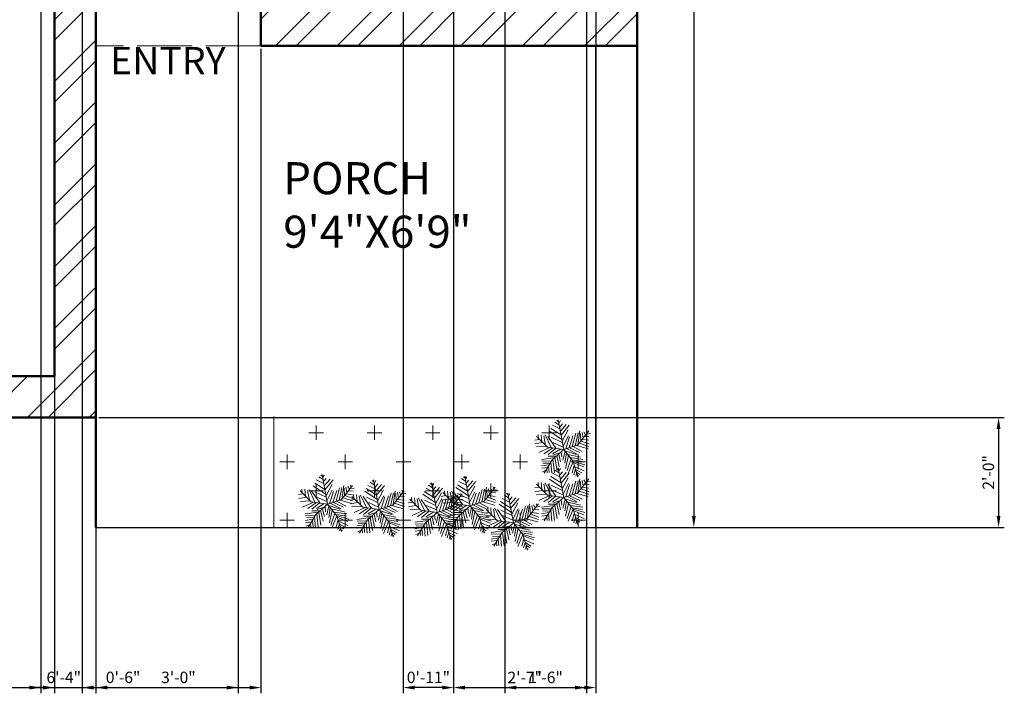
# Model space of a CAD drawing. Units: inches. Extents: x 1147 to 1568, y 1982 to 2559.
# Tile 2 of 4: x 1353 to 1568, y 1982 to 2128. Entities that reach past the tile are written whole.
import ezdxf

# ---------------------------------------------------------------- set-up
doc = ezdxf.new("R2010")
doc.units = ezdxf.units.IN
doc.linetypes.add('ACAD_ISO02W100', pattern=[15, 12, -3])
for name, color, linetype, lineweight in [('A-ANNO-DIMS', 2, 'Continuous', 18), ('A-FLOR', 7, 'Continuous', 25), ('A-WALL', 7, 'Continuous', 50), ('A-WALL-PATT', 252, 'Continuous', 13), ('L-PLNT', 3, 'Continuous', 18)]:
    doc.layers.add(name, color=color, linetype=linetype, lineweight=lineweight)
for name, color, linetype, lineweight, true_color in [('A-ANNO-TEXT', 244, 'Continuous', 18, 0x991b1e), ('A-AREA-IDEN', 244, 'Continuous', 25, 0x991b1e), ('A-WALL-OVHD', 244, 'ACAD_ISO02W100', 18, 0x991b1e), ('L-PLNT-PATT', 116, 'Continuous', 13, 0x136734)]:
    doc.layers.add(name, color=color, linetype=linetype, lineweight=lineweight, true_color=true_color)
doc.styles.get("Standard").update_dxf_attribs({"font": 'arial.ttf'})
doc.dimstyles.new('ISO-25', dxfattribs={"dimtxt": 2.5, "dimasz": 2.5, "dimexe": 1.25, "dimexo": 0.625, "dimtad": 1, "dimlunit": 3, "dimtxsty": 'Standard', "dimcen": 2.5, "dimadec": 0, "dimazin": 0, "dimtfac": 1, "dimtmove": 0, "dimatfit": 3, "dimfxl": 1, "dimarcsym": 0})

# ---------------------------------------------------------------- blocks, each defined once
blk = doc.blocks.new('*U8')
for p, q in [((0, 0), (-10.5, 57)), ((-5.114, 28.097), (-24.676, 40.636)), ((-7.288, 39.707), (-21.778, 46.673)), ((-8.737, 47.138), (-17.069, 52.711)), ((-10.186, 53.64), (-13.084, 55.962)), ((-9.099, 51.782), (-6.563, 55.962)), ((-7.65, 43.423), (-2.578, 49.46)), ((-5.839, 35.992), (4.667, 48.067)), ((-5.114, 27.632), (10.463, 46.673)), ((-2.941, 16.486), (8.652, 37.85)), ((-47.498, 19.737), (-55.83, 18.344)), ((-31.5, 4.5), (-52.5, 25.5)), ((-48.585, 21.131), (-49.309, 29.026)), ((-43.513, 28.561), (-42.427, 15.558)), ((-38.442, 26.239), (-34.819, 7.663)), ((-35.544, 28.097), (-24.314, 3.947)), ((-14.533, 2.09), (-30.834, 25.31)), ((-3.665, 19.273), (-27.574, 35.527)), ((-24.314, 23.917), (-2.941, 13.7)), ((-1.129, 6.734), (9.014, 26.704)), ((3.942, 1.625), (11.187, 24.381)), ((10.101, 3.483), (17.708, 26.239)), ((16.259, 5.805), (23.142, 31.348)), ((22.055, 7.198), (27.489, 32.277)), ((27, 9), (48, 36)), ((27.127, 9.056), (31.112, 35.992)), ((31.836, 30.883), (32.561, 16.486)), ((35.096, 32.741), (37.27, 22.524)), ((36.183, 19.737), (48.137, 17.88)), ((38.719, 34.134), (41.979, 28.561)), ((40.53, 25.775), (48.862, 24.846)), ((43.791, 29.954), (51.036, 30.883)), ((44.153, 36.456), (45.239, 32.741)), ((-40.615, 13.7), (-55.105, 10.913)), ((-33.37, 6.269), (-52.207, 5.34)), ((-28.299, 3.483), (-47.86, -5.805)), ((-21.416, 3.018), (-38.079, -8.128)), ((0, 0), (-31.5, 4.5)), ((-15.982, 2.09), (-30.11, -9.521)), ((0, 0), (-22.5, -19.5)), ((-6.563, 1.161), (-21.416, -8.128)), ((-20.691, 13.7), (-1.129, 4.876)), ((0, 0), (27, 9)), ((0, 0), (18, -22.5)), ((6.478, 1.625), (26.04, -8.592)), ((11.187, 3.483), (30.749, -5.805)), ((18.07, 5.805), (35.096, -3.483)), ((24.229, 7.663), (46.688, 1.625)), ((29.662, 12.307), (48.137, 6.269)), ((33.285, 16.486), (48.862, 10.913)), ((-17.431, -15.094), (-42.789, -18.809)), ((-15.257, -12.772), (-30.11, -12.772)), ((-20.691, -18.345), (-17.793, -44.352)), ((-6.563, -5.805), (-19.967, -9.985)), ((-17.069, -15.094), (-12.721, -40.172)), ((-13.446, -11.378), (-8.737, -32.741)), ((-9.461, -8.592), (-6.201, -23.453)), ((-4.752, -3.483), (-3.665, -14.629)), ((2.493, -3.019), (-1.491, -20.202)), ((1.769, -2.555), (24.229, -9.521)), ((5.029, -6.27), (2.131, -25.775)), ((9.014, -11.378), (3.58, -35.992)), ((14.085, -16.951), (6.478, -40.172)), ((7.565, -9.056), (32.198, -14.629)), ((12.274, -15.094), (36.907, -18.809)), ((-28.299, -29.026), (-42.789, -31.348)), ((-24.314, -21.596), (-42.427, -22.06)), ((-30.834, -34.135), (-42.427, -35.528)), ((-26.849, -26.24), (-40.253, -25.775)), ((-22.5, -19.5), (-37.5, -45)), ((-32.646, -36.921), (-31.921, -44.352)), ((-29.023, -30.884), (-27.936, -43.887)), ((-25.038, -23.918), (-22.865, -45.281)), ((18.07, -22.524), (8.289, -45.745)), ((20.244, -30.419), (15.897, -44.816)), ((16.259, -19.738), (36.183, -22.989)), ((18, -22.5), (27, -52.5)), ((18.433, -22.524), (40.53, -29.026)), ((19.157, -25.311), (38.719, -33.206)), ((21.331, -32.741), (39.081, -40.636)), ((-34.457, -39.708), (-40.978, -42.494)), ((22.78, -37.85), (19.519, -48.532)), ((22.78, -38.314), (34.372, -44.816)), ((24.591, -45.745), (23.142, -50.854)), ((24.591, -43.423), (30.749, -47.603)), ((26.764, -49.925), (28.213, -50.854))]:
    blk.add_line(p, q)
blk = doc.blocks.new('*D13')
at = {"layer": 'A-ANNO-DIMS', "color": 0, "lineweight": -2, "transparency": 16777216}
for p, q in [((1488.23, 2527.7), (1501.22, 2527.7)), ((1499.97, 2525.2), (1499.97, 2020.2)), ((1488.23, 2017.7), (1501.22, 2017.7))]:
    blk.add_line(p, q, dxfattribs=at)
at = {"layer": 'A-ANNO-DIMS', "color": 0, "transparency": 16777216}
for points in [[(1499.56, 2525.2), (1500.39, 2525.2), (1499.97, 2527.7)], [(1499.56, 2020.2), (1500.39, 2020.2), (1499.97, 2017.7)]]:
    blk.add_solid(points, dxfattribs=at)
at = {"layer": 'Defpoints', "color": 0, "transparency": 16777216}
for p in [(1487.61, 2527.7), (1487.61, 2017.7), (1499.97, 2017.7)]:
    blk.add_point(p, dxfattribs=at)
at = {"layer": 'A-ANNO-DIMS', "color": 0, "transparency": 16777216, "insert": (1498.07, 2272.7), "char_height": 2.5, "attachment_point": 5, "rotation": 90}
blk.add_mtext('42\'-6"', dxfattribs=at)
blk = doc.blocks.new('*D43')
at = {"layer": 'A-ANNO-DIMS', "color": 0, "lineweight": -2, "transparency": 16777216}
for p, q in [((1327.61, 2368.08), (1327.61, 1981.52)), ((1357.61, 2368.08), (1357.61, 1981.52)), ((1330.11, 1982.77), (1355.11, 1982.77))]:
    blk.add_line(p, q, dxfattribs=at)
at = {"layer": 'A-ANNO-DIMS', "color": 0, "transparency": 16777216}
for points in [[(1330.11, 1983.19), (1330.11, 1982.35), (1327.61, 1982.77)], [(1355.11, 1983.19), (1355.11, 1982.35), (1357.61, 1982.77)]]:
    blk.add_solid(points, dxfattribs=at)
at = {"layer": 'Defpoints', "color": 0, "transparency": 16777216}
for p in [(1327.61, 2368.7), (1357.61, 2368.7), (1357.61, 1982.77)]:
    blk.add_point(p, dxfattribs=at)
at = {"layer": 'A-ANNO-DIMS', "color": 0, "transparency": 16777216, "insert": (1342.61, 1984.67), "char_height": 2.5, "attachment_point": 5}
blk.add_mtext('2\'-6"', dxfattribs=at)
blk = doc.blocks.new('*D46')
at = {"layer": 'A-ANNO-DIMS', "color": 0, "lineweight": -2, "transparency": 16777216}
for p, q in [((1369.61, 2122.08), (1369.61, 1981.52)), ((1405.61, 2122.08), (1405.61, 1981.52)), ((1372.11, 1982.77), (1403.11, 1982.77))]:
    blk.add_line(p, q, dxfattribs=at)
at = {"layer": 'A-ANNO-DIMS', "color": 0, "transparency": 16777216}
for points in [[(1372.11, 1983.19), (1372.11, 1982.35), (1369.61, 1982.77)], [(1403.11, 1983.19), (1403.11, 1982.35), (1405.61, 1982.77)]]:
    blk.add_solid(points, dxfattribs=at)
at = {"layer": 'Defpoints', "color": 0, "transparency": 16777216}
for p in [(1369.61, 2122.7), (1405.61, 2122.7), (1405.61, 1982.77)]:
    blk.add_point(p, dxfattribs=at)
at = {"layer": 'A-ANNO-DIMS', "color": 0, "transparency": 16777216, "insert": (1387.61, 1984.67), "char_height": 2.5, "attachment_point": 5}
blk.add_mtext('3\'-0"', dxfattribs=at)
blk = doc.blocks.new('*D47')
at = {"layer": 'A-ANNO-DIMS', "color": 0, "lineweight": -2, "transparency": 16777216}
for p, q in [((1436.61, 2166.08), (1436.61, 1981.52)), ((1447.61, 2166.08), (1447.61, 1981.52)), ((1445.11, 1982.77), (1439.11, 1982.77))]:
    blk.add_line(p, q, dxfattribs=at)
at = {"layer": 'A-ANNO-DIMS', "color": 0, "transparency": 16777216}
for points in [[(1439.11, 1983.19), (1439.11, 1982.35), (1436.61, 1982.77)], [(1445.11, 1983.19), (1445.11, 1982.35), (1447.61, 1982.77)]]:
    blk.add_solid(points, dxfattribs=at)
at = {"layer": 'Defpoints', "color": 0, "transparency": 16777216}
for p in [(1436.61, 2166.7), (1447.61, 2166.7), (1436.61, 1982.77)]:
    blk.add_point(p, dxfattribs=at)
at = {"layer": 'A-ANNO-DIMS', "color": 0, "transparency": 16777216, "insert": (1442.11, 1984.67), "char_height": 2.5, "attachment_point": 5}
blk.add_mtext('0\'-11"', dxfattribs=at)
blk = doc.blocks.new('*D49')
at = {"layer": 'A-ANNO-DIMS', "color": 0, "lineweight": -2, "transparency": 16777216}
for p, q in [((1447.61, 2131.08), (1447.61, 1981.52)), ((1478.61, 2131.08), (1478.61, 1981.52)), ((1450.11, 1982.77), (1476.11, 1982.77))]:
    blk.add_line(p, q, dxfattribs=at)
at = {"layer": 'A-ANNO-DIMS', "color": 0, "transparency": 16777216}
for points in [[(1450.11, 1983.19), (1450.11, 1982.35), (1447.61, 1982.77)], [(1476.11, 1983.19), (1476.11, 1982.35), (1478.61, 1982.77)]]:
    blk.add_solid(points, dxfattribs=at)
at = {"layer": 'Defpoints', "color": 0, "transparency": 16777216}
for p in [(1447.61, 2131.7), (1478.61, 2131.7), (1478.61, 1982.77)]:
    blk.add_point(p, dxfattribs=at)
at = {"layer": 'A-ANNO-DIMS', "color": 0, "transparency": 16777216, "insert": (1463.11, 1984.65), "char_height": 2.5, "attachment_point": 5}
blk.add_mtext('2\'-7"', dxfattribs=at)
blk = doc.blocks.new('*D51')
at = {"layer": 'A-ANNO-DIMS', "color": 0, "lineweight": -2, "transparency": 16777216}
for p, q in [((1360.61, 2518.08), (1360.61, 1981.52)), ((1366.61, 2518.08), (1366.61, 1981.52)), ((1358.11, 1982.77), (1355.61, 1982.77)), ((1360.61, 1982.77), (1366.61, 1982.77)), ((1369.11, 1982.77), (1379.5, 1982.77))]:
    blk.add_line(p, q, dxfattribs=at)
at = {"layer": 'A-ANNO-DIMS', "color": 0, "transparency": 16777216}
for points in [[(1358.11, 1983.19), (1358.11, 1982.35), (1360.61, 1982.77)], [(1369.11, 1983.19), (1369.11, 1982.35), (1366.61, 1982.77)]]:
    blk.add_solid(points, dxfattribs=at)
at = {"layer": 'Defpoints', "color": 0, "transparency": 16777216}
for p in [(1360.61, 2518.7), (1366.61, 2518.7), (1366.61, 1982.77)]:
    blk.add_point(p, dxfattribs=at)
at = {"layer": 'A-ANNO-DIMS', "color": 0, "transparency": 16777216, "insert": (1375.55, 1984.67), "char_height": 2.5, "attachment_point": 5}
blk.add_mtext('0\'-6"', dxfattribs=at)
blk = doc.blocks.new('*D56')
at = {"layer": 'A-ANNO-DIMS', "color": 0, "lineweight": -2, "transparency": 16777216}
for p, q in [((1370.23, 2041.7), (1567.66, 2041.7)), ((1566.41, 2039.2), (1566.41, 2020.2)), ((1370.23, 2017.7), (1567.66, 2017.7))]:
    blk.add_line(p, q, dxfattribs=at)
at = {"layer": 'A-ANNO-DIMS', "color": 0, "transparency": 16777216}
for points in [[(1565.99, 2039.2), (1566.82, 2039.2), (1566.41, 2041.7)], [(1565.99, 2020.2), (1566.82, 2020.2), (1566.41, 2017.7)]]:
    blk.add_solid(points, dxfattribs=at)
at = {"layer": 'Defpoints', "color": 0, "transparency": 16777216}
for p in [(1369.61, 2041.7), (1369.61, 2017.7), (1566.41, 2017.7)]:
    blk.add_point(p, dxfattribs=at)
at = {"layer": 'A-ANNO-DIMS', "color": 0, "transparency": 16777216, "insert": (1564.51, 2029.7), "char_height": 2.5, "attachment_point": 5, "rotation": 90}
blk.add_mtext('2\'-0"', dxfattribs=at)
blk = doc.blocks.new('*D62')
at = {"layer": 'A-ANNO-DIMS', "color": 0, "lineweight": -2, "transparency": 16777216}
for p, q in [((1324.61, 2335.08), (1324.61, 1981.52)), ((1400.61, 2335.08), (1400.61, 1981.52)), ((1327.11, 1982.77), (1398.11, 1982.77))]:
    blk.add_line(p, q, dxfattribs=at)
at = {"layer": 'A-ANNO-DIMS', "color": 0, "transparency": 16777216}
for points in [[(1327.11, 1983.19), (1327.11, 1982.35), (1324.61, 1982.77)], [(1398.11, 1983.19), (1398.11, 1982.35), (1400.61, 1982.77)]]:
    blk.add_solid(points, dxfattribs=at)
at = {"layer": 'Defpoints', "color": 0, "transparency": 16777216}
for p in [(1324.61, 2335.7), (1400.61, 2335.7), (1400.61, 1982.77)]:
    blk.add_point(p, dxfattribs=at)
at = {"layer": 'A-ANNO-DIMS', "color": 0, "transparency": 16777216, "insert": (1362.61, 1984.67), "char_height": 2.5, "attachment_point": 5}
blk.add_mtext('6\'-4"', dxfattribs=at)
blk = doc.blocks.new('*D65')
at = {"layer": 'A-ANNO-DIMS', "color": 0, "lineweight": -2, "transparency": 16777216}
for p, q in [((1458.78, 2235.1), (1458.78, 1981.52)), ((1476.55, 2235.16), (1476.55, 1981.52)), ((1461.28, 1982.77), (1474.05, 1982.77))]:
    blk.add_line(p, q, dxfattribs=at)
at = {"layer": 'A-ANNO-DIMS', "color": 0, "transparency": 16777216}
for points in [[(1461.28, 1983.19), (1461.28, 1982.35), (1458.78, 1982.77)], [(1474.05, 1983.19), (1474.05, 1982.35), (1476.55, 1982.77)]]:
    blk.add_solid(points, dxfattribs=at)
at = {"layer": 'Defpoints', "color": 0, "transparency": 16777216}
for p in [(1458.78, 2235.73), (1476.55, 2235.78), (1476.55, 1982.77)]:
    blk.add_point(p, dxfattribs=at)
at = {"layer": 'A-ANNO-DIMS', "color": 0, "transparency": 16777216, "insert": (1467.66, 1984.67), "char_height": 2.5, "attachment_point": 5}
blk.add_mtext('1\'-6"', dxfattribs=at)

msp = doc.modelspace()

# ---------------------------------------------------------------- hatches: boundary and pattern name
at = {"layer": 'A-WALL-PATT'}
h = msp.add_hatch(dxfattribs=at)
h.set_pattern_fill('ANSI32', color=256)
h.paths.add_polyline_path([(1240.607, 2518.704), (1268.63, 2518.704), (1268.63, 2527.704), (1231.607, 2527.704), (1231.607, 2348.295), (1240.607, 2348.295), (1240.607, 2368.704), (1318.607, 2368.704), (1318.607, 2365.704), (1324.607, 2365.704), (1324.607, 2368.704), (1327.607, 2368.704), (1327.607, 2374.704), (1240.607, 2374.704)])
h.paths.add_polyline_path([(1324.607, 2335.704), (1318.607, 2335.704), (1318.607, 2314.704), (1240.607, 2314.704), (1240.607, 2324.295), (1231.607, 2324.295), (1231.607, 2247.419), (1240.607, 2247.419), (1240.607, 2308.704), (1324.607, 2308.704)])
h.paths.add_polyline_path([(1487.607, 2527.704), (1464.679, 2527.704), (1464.679, 2518.704), (1478.607, 2518.704), (1478.607, 2374.704), (1399.607, 2374.704), (1399.607, 2368.704), (1400.607, 2368.704), (1400.607, 2365.704), (1406.607, 2365.704), (1406.607, 2368.704), (1478.607, 2368.704), (1478.607, 2343.549), (1487.607, 2343.549)])
h.paths.add_polyline_path([(1366.607, 2518.704), (1398.679, 2518.704), (1398.679, 2527.704), (1334.63, 2527.704), (1334.63, 2518.704), (1360.607, 2518.704), (1360.607, 2374.704), (1357.607, 2374.704), (1357.607, 2368.704), (1369.607, 2368.704), (1369.607, 2374.704), (1366.607, 2374.704)])
h.paths.add_polyline_path([(1487.607, 2319.549), (1478.607, 2319.549), (1478.607, 2314.704), (1406.607, 2314.704), (1406.607, 2335.704), (1400.607, 2335.704), (1400.607, 2308.704), (1406.607, 2308.704), (1406.607, 2284.704), (1412.607, 2284.704), (1412.607, 2308.704), (1478.607, 2308.704), (1478.607, 2295.917), (1487.607, 2295.917)])
h.paths.add_polyline_path([(1487.607, 2235.917), (1478.607, 2235.917), (1478.607, 2212.704), (1400.607, 2212.704), (1400.607, 2206.704), (1478.607, 2206.704), (1478.607, 2131.704), (1405.607, 2131.704), (1405.607, 2122.704), (1487.607, 2122.704)])
h.paths.add_polyline_path([(1369.607, 2122.704), (1369.607, 2131.704), (1366.607, 2131.704), (1366.607, 2176.704), (1357.607, 2176.704), (1357.607, 2170.704), (1360.607, 2170.704), (1360.607, 2050.704), (1334.63, 2050.704), (1334.63, 2041.704), (1369.607, 2041.704)])
h.paths.add_polyline_path([(1240.607, 2170.704), (1321.607, 2170.704), (1321.607, 2176.704), (1240.607, 2176.704), (1240.607, 2187.419), (1231.607, 2187.419), (1231.607, 2041.704), (1268.63, 2041.704), (1268.63, 2050.704), (1240.607, 2050.704)])
at = {"layer": 'L-PLNT-PATT'}
h = msp.add_hatch(dxfattribs=at)
h.set_pattern_fill('CROSS', color=256)
h.paths.add_polyline_path([(1478.607, 2041.704), (1408.398, 2041.704), (1408.398, 2017.704), (1478.607, 2017.704)])
h.paths.add_polyline_path([(1431.023, 2023.435), (1431.134, 2023.64), (1430.963, 2023.756)], flags=16)
h.paths.add_polyline_path([(1436.583, 2025.011), (1436.507, 2025.271), (1436.274, 2024.971)], flags=16)
h.paths.add_polyline_path([(1431.899, 2020.624), (1432.179, 2020.56), (1431.935, 2020.865)], flags=16)
h.paths.add_polyline_path([(1430.596, 2020.912), (1430.247, 2020.803), (1430.282, 2020.641)], flags=16)
h.paths.add_polyline_path([(1420.698, 2022.051), (1420.662, 2021.809), (1420.942, 2021.746)], flags=16)
h.paths.add_polyline_path([(1417.744, 2020.991), (1417.773, 2020.724), (1418.15, 2021.051)], flags=16)
h.paths.add_polyline_path([(1418.479, 2023), (1418.417, 2023.087), (1418.336, 2023.02)], flags=16)
h.paths.add_polyline_path([(1419.056, 2028.579), (1419.14, 2028.718), (1419.011, 2028.821)], flags=16)
h.paths.add_polyline_path([(1425.346, 2026.196), (1425.27, 2026.457), (1425.036, 2026.157)], flags=16)
h.paths.add_polyline_path([(1429.716, 2021.814), (1429.655, 2021.901), (1429.573, 2021.834)], flags=16)
h.paths.add_polyline_path([(1434.409, 2022.369), (1434.444, 2022.605), (1434.037, 2022.469)], flags=16)
h.paths.add_polyline_path([(1442.357, 2021.181), (1442.296, 2021.269), (1442.214, 2021.202)], flags=16)
h.paths.add_polyline_path([(1438.485, 2023.401), (1440.229, 2021.658), (1440.085, 2021.651), (1440.049, 2021.838), (1439.387, 2022.5), (1439.21, 2022.465), (1439.191, 2022.696), (1438.688, 2023.199), (1438.507, 2023.168)], flags=16)
h.paths.add_polyline_path([(1442.935, 2026.761), (1443.019, 2026.9), (1442.89, 2027.003)], flags=16)
h.paths.add_polyline_path([(1450.159, 2028.21), (1450.243, 2028.349), (1450.115, 2028.452)], flags=16)
h.paths.add_polyline_path([(1448.683, 2024.04), (1448.921, 2023.932), (1448.783, 2024.169)], flags=16)
h.paths.add_polyline_path([(1456.449, 2025.827), (1456.373, 2026.088), (1456.139, 2025.788)], flags=16)
h.paths.add_polyline_path([(1454.275, 2023.186), (1454.31, 2023.421), (1453.903, 2023.286)], flags=16)
h.paths.add_polyline_path([(1459.569, 2024.548), (1459.653, 2024.686), (1459.525, 2024.789)], flags=16)
h.paths.add_polyline_path([(1465.859, 2022.165), (1465.783, 2022.425), (1465.55, 2022.125)], flags=16)
h.paths.add_polyline_path([(1463.685, 2019.523), (1463.72, 2019.759), (1463.313, 2019.623)], flags=16)
h.paths.add_polyline_path([(1451.801, 2021.682), (1451.765, 2021.44), (1452.045, 2021.377)], flags=16)
h.paths.add_polyline_path([(1444.577, 2020.232), (1444.541, 2019.991), (1444.82, 2019.928)], flags=16)
h.paths.add_polyline_path([(1442.888, 2020.171), (1442.924, 2020.008), (1443.237, 2020.279)], flags=16)
h.paths.add_polyline_path([(1446.917, 2023.643), (1447.068, 2024.34), (1447.273, 2023.287), (1447.279, 2023.281), (1447.517, 2024.892), (1448.326, 2023.153), (1449.324, 2022.998), (1449.582, 2022.631), (1451.23, 2022.395), (1450.697, 2021.933), (1450.71, 2021.806), (1450.461, 2021.729), (1449.71, 2021.077), (1449.739, 2020.945), (1449.557, 2020.945), (1449.288, 2020.711), (1449.292, 2020.687), (1446.4, 2020.264), (1444.67, 2021.167), (1444.441, 2021.091), (1445.269, 2023.69), (1446.435, 2023.915), (1446.415, 2024.145), (1445.912, 2024.648), (1445.731, 2024.618), (1445.71, 2024.851)], flags=16)
h.paths.add_polyline_path([(1427.587, 2022.291), (1427.444, 2022.284), (1427.407, 2022.47), (1426.746, 2023.132), (1425.579, 2022.908), (1422.8, 2023.655), (1420.562, 2022.909), (1420.616, 2023.078), (1420.792, 2022.986), (1421.269, 2023.145), (1421.291, 2023.21), (1421.363, 2023.176), (1421.96, 2023.375), (1421.999, 2023.521), (1422.15, 2023.438), (1422.635, 2023.6), (1422.655, 2023.694), (1422.8, 2023.655), (1423.206, 2023.791), (1423.272, 2024.234), (1425.026, 2023.661), (1425.865, 2023.801), (1425.844, 2024.034)], flags=16)
h.paths.add_polyline_path([(1447.687, 2023.119), (1447.701, 2022.847), (1449.798, 2022.097), (1448.569, 2021.328), (1447.23, 2021.688), (1446.635, 2021.29), (1445.808, 2021.741), (1445.9, 2021.785), (1446.24, 2023.047)], flags=0)
h.paths.add_polyline_path([(1449.837, 2024.457), (1449.225, 2024.378), (1449.099, 2024.81)], flags=16)
h.paths.add_polyline_path([(1416.35, 2023.476), (1416.207, 2023.469), (1416.17, 2023.656), (1415.508, 2024.318), (1415.331, 2024.284), (1415.312, 2024.514), (1414.809, 2025.017), (1414.628, 2024.987), (1414.606, 2025.22)], flags=16)
h.paths.add_polyline_path([(1455.12, 2021.188), (1457.065, 2019.243), (1458.215, 2019.079), (1457.996, 2018.932), (1457.907, 2019.123), (1457.531, 2019.177), (1457.26, 2019.048), (1456.863, 2019.445), (1456.72, 2019.438), (1456.684, 2019.624), (1456.022, 2020.286), (1455.845, 2020.252), (1455.825, 2020.482), (1455.322, 2020.985), (1455.141, 2020.955)], flags=16)
h.paths.add_polyline_path([(1469.971, 2034.901), (1469.909, 2034.989), (1469.828, 2034.922)], flags=16)
h.paths.add_polyline_path([(1466.823, 2036.185), (1466.804, 2036.416), (1466.301, 2036.919), (1466.12, 2036.888), (1466.098, 2037.121), (1467.842, 2035.378), (1467.699, 2035.371), (1467.662, 2035.558), (1467, 2036.219)], flags=16)
h.paths.add_polyline_path([(1469.971, 2024.458), (1469.909, 2024.546), (1469.828, 2024.479)], flags=16)
h.paths.add_polyline_path([(1466.12, 2026.445), (1466.098, 2026.678), (1467.842, 2024.935), (1467.699, 2024.928), (1467.662, 2025.115), (1467, 2025.776), (1466.823, 2025.742), (1466.804, 2025.973), (1466.301, 2026.476)], flags=16)
h.paths.add_polyline_path([(1469.946, 2033.216), (1469.636, 2033.216), (1469.676, 2032.982)], flags=16)
h.paths.add_polyline_path([(1470.548, 2030.038), (1470.632, 2030.176), (1470.503, 2030.279)], flags=16)
h.paths.add_polyline_path([(1468.926, 2032.216), (1468.75, 2032.211), (1468.776, 2031.96)], flags=16)
h.paths.add_polyline_path([(1469.946, 2022.773), (1469.636, 2022.773), (1469.676, 2022.539)], flags=16)
h.paths.add_polyline_path([(1468.085, 2020.343), (1467.885, 2020.319), (1467.911, 2020.048)], flags=16)
h.paths.add_polyline_path([(1470.548, 2040.481), (1470.632, 2040.62), (1470.503, 2040.723)], flags=16)
h.paths.add_polyline_path([(1472.19, 2033.952), (1472.154, 2033.711), (1472.434, 2033.648)], flags=16)
h.paths.add_polyline_path([(1476.838, 2038.098), (1476.762, 2038.359), (1476.528, 2038.058)], flags=16)
h.paths.add_polyline_path([(1474.664, 2035.457), (1474.698, 2035.692), (1474.292, 2035.557)], flags=16)
h.paths.add_polyline_path([(1476.838, 2027.655), (1476.762, 2027.915), (1476.528, 2027.615)], flags=16)
h.paths.add_polyline_path([(1474.664, 2025.014), (1474.698, 2025.249), (1474.292, 2025.113)], flags=16)
h.paths.add_polyline_path([(1474.195, 2019.893), (1474.191, 2019.881), (1474.2, 2019.876)], flags=16)
h.paths.add_polyline_path([(1472.19, 2023.509), (1472.154, 2023.268), (1472.434, 2023.205)], flags=16)
h.paths.add_polyline_path([(1474.195, 2030.336), (1474.191, 2030.324), (1474.2, 2030.319)], flags=16)

# ---------------------------------------------------------------- linework, layer by layer
at = {"layer": 'A-FLOR'}
for p, q in [((1478.607, 2017.704), (1478.607, 2122.704)), ((1369.607, 2017.704), (1487.607, 2017.704))]:
    msp.add_line(p, q, dxfattribs=at)
at = {"layer": 'A-WALL'}
for p, q in [((1487.607, 2017.704), (1487.607, 2527.704)), ((1360.607, 2050.704), (1360.607, 2170.704)), ((1369.607, 2122.704), (1369.607, 2131.704)), ((1405.607, 2122.704), (1405.607, 2131.704)), ((1369.607, 2017.704), (1369.607, 2122.704)), ((1405.607, 2122.704), (1487.607, 2122.704)), ((1240.607, 2050.704), (1360.607, 2050.704)), ((1231.607, 2041.704), (1369.607, 2041.704))]:
    msp.add_line(p, q, dxfattribs=at)
at = {"layer": 'A-WALL-OVHD'}
msp.add_line((1405.607, 2122.704), (1369.607, 2122.704), dxfattribs=at)
at = {"layer": 'L-PLNT'}
for p, q in [((1408.398, 2041.897), (1408.398, 2017.704)), ((1408.398, 2041.704), (1478.607, 2041.704))]:
    msp.add_line(p, q, dxfattribs=at)

# ---------------------------------------------------------------- block references
at = {"layer": 'L-PLNT', "xscale": 0.1135232311302616, "yscale": 0.1135232311302616, "zscale": 0.1135232311302616}
for p in [(1471.619, 2034.666), (1471.619, 2024.223), (1420.127, 2022.764), (1451.23, 2022.395), (1431.365, 2021.578), (1444.006, 2020.946), (1460.641, 2018.732)]:
    msp.add_blockref('*U8', p, dxfattribs=at)

# ---------------------------------------------------------------- texts
at = {"layer": 'A-ANNO-TEXT', "insert": (1372.714, 2122.499), "char_height": 6, "attachment_point": 1}
msp.add_mtext_dynamic_manual_height_columns('{ENTRY}', width=27.74603, gutter_width=12.5, heights=[0], dxfattribs=at)
at = {"layer": 'A-AREA-IDEN', "insert": (1410.471, 2097.357), "char_height": 7, "attachment_point": 1}
msp.add_mtext_dynamic_manual_height_columns('{PORCH\\P9\'4"X6\'9"}', width=38.23855, gutter_width=12.5, heights=[0], dxfattribs=at)

# ---------------------------------------------------------------- dimensions: what is measured, and where the dimension line sits
at = {"layer": 'A-ANNO-DIMS'}
for base, p1, p2, override, picture, middle in [((1499.975, 2017.704), (1487.607, 2527.704), (1487.607, 2017.704), {"dimclrd": 0, "dimclre": 0, "dimclrt": 0}, '*D13', (1498.073, 2272.704)), ((1566.407, 2017.704), (1369.607, 2041.704), (1369.607, 2017.704), {"dimdec": 1, "dimlfac": 1, "dimrnd": 0, "dimzin": 1, "dimdsep": 46, "dimlunit": 4, "dimfrac": 2}, '*D56', (1564.505, 2029.704))]:
    dim = msp.add_linear_dim(base=base, p1=p1, p2=p2, angle=90, dimstyle='ISO-25', override=override, dxfattribs=at)
    dim.commit()
    dim.dimension.update_dxf_attribs({"geometry": picture, "text_midpoint": middle})
for base, p1, p2, picture, middle in [((1366.607, 1982.772), (1360.607, 2518.704), (1366.607, 2518.704), '*D51', (1375.555, 1984.673)), ((1357.607, 1982.772), (1327.607, 2368.704), (1357.607, 2368.704), '*D43', (1342.607, 1984.673)), ((1400.607, 1982.772), (1324.607, 2335.704), (1400.607, 2335.704), '*D62', (1362.607, 1984.673)), ((1476.551, 1982.772), (1458.779, 2235.728), (1476.551, 2235.784), '*D65', (1467.665, 1984.673)), ((1436.607, 1982.772), (1447.607, 2166.704), (1436.607, 2166.704), '*D47', (1442.107, 1984.673)), ((1478.607, 1982.772), (1447.607, 2131.704), (1478.607, 2131.704), '*D49', (1463.107, 1984.652)), ((1405.607, 1982.772), (1369.607, 2122.704), (1405.607, 2122.704), '*D46', (1387.607, 1984.674))]:
    dim = msp.add_linear_dim(base=base, p1=p1, p2=p2, dimstyle='ISO-25', override={"dimdec": 1, "dimlfac": 1, "dimrnd": 0, "dimzin": 1, "dimdsep": 46, "dimlunit": 4, "dimfrac": 2}, dxfattribs=at)
    dim.commit()
    dim.dimension.update_dxf_attribs({"geometry": picture, "text_midpoint": middle})

doc.saveas('drawing.dxf')
